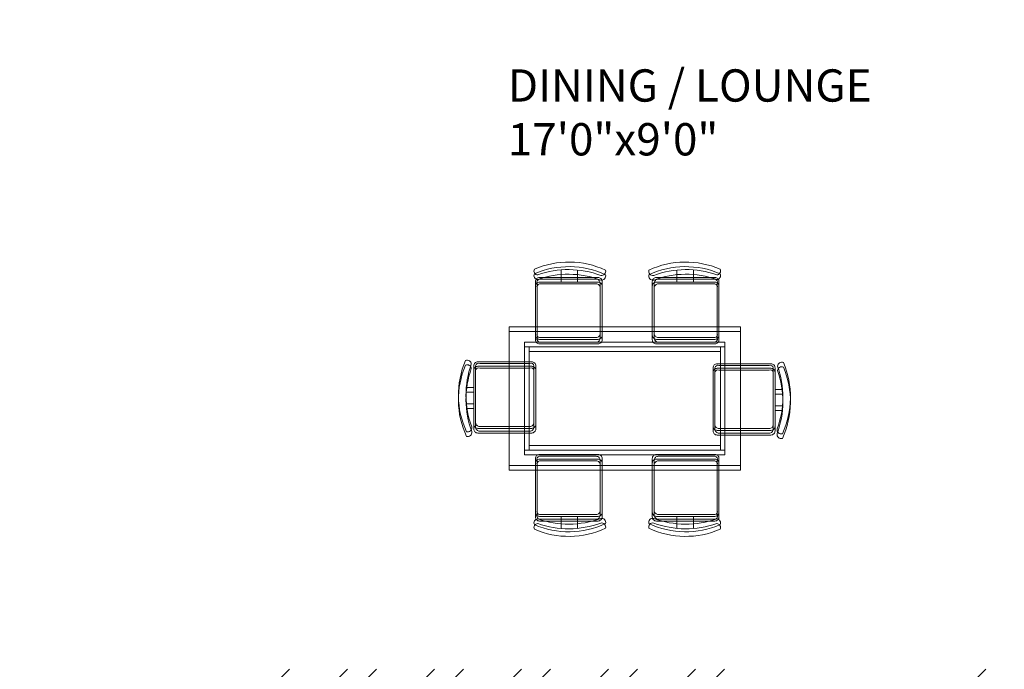
# Model space of a CAD drawing. Units: inches. Extents: x 963 to 2075, y 289 to 2657.
# Tile 55 of 98: x 1663 to 1815, y 1714 to 1814. Entities that reach past the tile are written whole.
import ezdxf

# ---------------------------------------------------------------- set-up
doc = ezdxf.new("R2010")
doc.units = ezdxf.units.IN
for name, color, linetype, lineweight in [('A-AREA-IDEN', 7, 'Continuous', 18), ('A-FURN', 8, 'Continuous', 18), ('A-WALL-PATT', 8, 'Continuous', 13)]:
    doc.layers.add(name, color=color, linetype=linetype, lineweight=lineweight)
doc.styles.get("Standard").update_dxf_attribs({"font": 'arial.ttf'})

msp = doc.modelspace()

# ---------------------------------------------------------------- hatches: boundary and pattern name
at = {"layer": 'A-WALL-PATT'}
h = msp.add_hatch(dxfattribs=at)
h.set_pattern_fill('ANSI32', color=256)
h.paths.add_polyline_path([(1296.92, 2558.32), (1203.92, 2558.32), (1203.92, 2493.82), (1191.53, 2493.82), (1191.53, 2489.32), (1211.06, 2489.32), (1211.06, 2492.02), (1211.06, 2493.82), (1208.42, 2493.82), (1208.42, 2553.82), (1292.42, 2553.82), (1292.42, 2538.86), (1296.92, 2538.86)])
h.paths.add_polyline_path([(1442.42, 2558.32), (1349.42, 2558.32), (1349.42, 2538.94), (1353.92, 2538.94), (1353.92, 2553.82), (1437.92, 2553.82), (1437.92, 2493.82), (1434.54, 2493.82), (1434.54, 2489.32), (1448.31, 2489.32), (1448.31, 2491.57), (1448.31, 2493.82), (1442.42, 2493.82)])
h.paths.add_polyline_path([(1415.55, 2491.57), (1415.55, 2493.82), (1340.94, 2493.82), (1340.94, 2489.32), (1371.92, 2489.32), (1371.92, 2378.32), (1367.6, 2378.32), (1367.6, 2373.82), (1371.92, 2373.82), (1371.92, 2355.19), (1376.42, 2355.19), (1376.42, 2489.32), (1415.55, 2489.32)])
h.paths.add_polyline_path([(1304.94, 2491.57), (1304.94, 2493.82), (1296.92, 2493.82), (1296.92, 2514.86), (1292.42, 2514.86), (1292.42, 2493.82), (1232.81, 2493.82), (1232.81, 2489.32), (1256.42, 2489.32), (1256.42, 2327.32), (1253.71, 2327.32), (1253.71, 2322.82), (1328.42, 2322.82), (1328.42, 2331.15), (1323.92, 2331.15), (1323.92, 2327.32), (1260.92, 2327.32), (1260.92, 2373.82), (1323.92, 2373.82), (1323.92, 2357.81), (1328.42, 2357.81), (1328.42, 2373.82), (1346.01, 2373.82), (1346.01, 2376.07), (1346.01, 2378.32), (1260.92, 2378.32), (1260.92, 2489.32), (1304.94, 2489.32)])
h.paths.add_polyline_path([(1226.65, 2327.32), (1124.42, 2327.32), (1124.42, 2347.45), (1119.92, 2347.45), (1119.92, 2322.82), (1163.42, 2322.82), (1163.42, 2305.43), (1165.67, 2305.43), (1167.92, 2305.43), (1167.92, 2322.82), (1226.65, 2322.82), (1226.65, 2325.07)])
h.paths.add_polyline_path([(1095.92, 2489.32), (1124.42, 2489.32), (1131.53, 2489.32), (1131.53, 2491.57), (1131.53, 2493.82), (1119.92, 2493.82), (1091.42, 2493.82), (1091.42, 2417.32), (1095.92, 2417.32), (1119.92, 2417.32), (1119.92, 2407.45), (1124.42, 2407.45), (1124.42, 2421.82), (1095.92, 2421.82)])
h.paths.add_polyline_path([(1512.92, 2558.32), (1508.42, 2558.32), (1508.42, 2493.82), (1503.4, 2493.82), (1503.4, 2489.32), (1508.42, 2489.32), (1508.42, 2327.32), (1376.42, 2327.32), (1376.42, 2330.27), (1371.92, 2330.27), (1371.92, 2298.74), (1376.42, 2298.74), (1376.42, 2322.82), (1508.42, 2322.82), (1508.42, 2165.32), (1504.26, 2165.32), (1504.26, 2160.82), (1508.42, 2160.82), (1508.42, 2108.32), (1512.92, 2108.32), (1512.92, 2160.82), (1516.18, 2160.82), (1516.18, 2163.07), (1516.18, 2165.32), (1512.92, 2165.32), (1512.92, 2322.82), (1644.92, 2322.82), (1644.92, 2298.74), (1649.42, 2298.74), (1649.42, 2322.82), (1649.42, 2330.94), (1647.17, 2330.94), (1644.92, 2330.94), (1644.92, 2327.32), (1512.92, 2327.32), (1512.92, 2489.32), (1516.76, 2489.32), (1516.76, 2491.57), (1516.76, 2493.82), (1512.92, 2493.82)])
h.paths.add_polyline_path([(1671.92, 2558.32), (1578.92, 2558.32), (1578.92, 2493.82), (1573.53, 2493.82), (1573.53, 2489.32), (1586.54, 2489.32), (1586.54, 2491.57), (1586.54, 2493.82), (1583.42, 2493.82), (1583.42, 2553.82), (1667.42, 2553.82), (1667.42, 2541.11), (1671.92, 2541.11)])
h.paths.add_polyline_path([(1681.26, 2493.82), (1671.92, 2493.82), (1671.92, 2517.11), (1667.42, 2517.11), (1667.42, 2493.82), (1610.22, 2493.82), (1610.22, 2489.32), (1644.92, 2489.32), (1644.92, 2357.87), (1649.42, 2357.87), (1649.42, 2373.82), (1652.2, 2373.82), (1652.2, 2375.83), (1652.2, 2378.32), (1649.42, 2378.32), (1649.42, 2489.32), (1681.26, 2489.32), (1681.26, 2491.57)])
h.paths.add_polyline_path([(1821.92, 2558.32), (1728.92, 2558.32), (1728.92, 2541), (1733.42, 2541), (1733.42, 2553.82), (1817.42, 2553.82), (1817.42, 2493.82), (1813.51, 2493.82), (1813.51, 2489.32), (1830.08, 2489.32), (1830.08, 2491.57), (1830.08, 2493.82), (1821.92, 2493.82)])
h.paths.add_polyline_path([(1794.24, 2493.82), (1717.26, 2493.82), (1717.26, 2489.32), (1760.42, 2489.32), (1760.42, 2378.32), (1674.4, 2378.32), (1674.4, 2373.82), (1692.92, 2373.82), (1692.92, 2356.95), (1697.42, 2356.95), (1697.42, 2373.82), (1760.42, 2373.82), (1760.42, 2327.32), (1697.42, 2327.32), (1697.42, 2333.34), (1692.92, 2333.34), (1692.92, 2322.82), (1768.04, 2322.82), (1768.04, 2325.07), (1768.04, 2327.32), (1764.92, 2327.32), (1764.92, 2489.32), (1794.24, 2489.32)])
h.paths.add_polyline_path([(1733.42, 2517), (1728.92, 2517), (1728.92, 2493.82), (1733.42, 2493.82)], flags=17)
h.paths.add_polyline_path([(1929.92, 2493.82), (1890.08, 2493.82), (1890.08, 2489.32), (1896.92, 2489.32), (1925.42, 2489.32), (1925.42, 2421.82), (1896.92, 2421.82), (1896.92, 2408.32), (1901.42, 2408.32), (1901.42, 2417.32), (1925.42, 2417.32), (1929.92, 2417.32)])
h.paths.add_polyline_path([(1901.42, 2348.32), (1896.92, 2348.32), (1896.92, 2327.32), (1800.42, 2327.32), (1800.42, 2322.82), (1853.42, 2322.82), (1853.42, 2309.45), (1857.92, 2309.45), (1857.92, 2322.82), (1901.42, 2322.82)])
h.paths.add_polyline_path([(1857.92, 2249.45), (1853.42, 2249.45), (1853.42, 2214.82), (1686.31, 2214.82), (1686.31, 2210.32), (1853.42, 2210.32), (1853.42, 2202.13), (1857.92, 2202.13), (1857.92, 2210.32)])
h.paths.add_polyline_path([(1857.92, 2142.13), (1853.42, 2142.13), (1853.42, 2115.42), (1841.42, 2115.42), (1841.42, 2088.53), (1841.42, 2046.95), (1845.92, 2046.95), (1845.92, 2110.92), (1905.92, 2110.92), (1905.92, 2092.52), (1910.42, 2092.52), (1910.42, 2115.42), (1857.92, 2115.42)])
h.paths.add_polyline_path([(1532.44, 1482.34), (1573.46, 1482.34), (1573.46, 1501), (1532.44, 1501)], flags=9)
h.paths.add_polyline_path([(1438.66, 1486.3), (1479.68, 1486.3), (1479.68, 1504.96), (1438.66, 1504.96)], flags=9)
h.paths.add_polyline_path([(1411.22, 1365.31), (1659.14, 1365.31), (1659.14, 1402.4), (1411.22, 1402.4)], flags=9)
h.paths.add_polyline_path([(1185.67, 2296.3), (1248.16, 2296.3), (1248.16, 2314.95), (1185.67, 2314.95)], flags=9)
h.paths.add_polyline_path([(1177.31, 2187.35), (1216.15, 2187.35), (1216.15, 2206.01), (1177.31, 2206.01)], flags=9)
h.paths.add_polyline_path([(1295.1, 1602.08), (1328.26, 1602.08), (1328.26, 1620.74), (1295.1, 1620.74)], flags=9)
h.paths.add_polyline_path([(1525.13, 2005.99), (1558.39, 2005.99), (1558.39, 2024.65), (1525.13, 2024.65)], flags=9)
h.paths.add_polyline_path([(1459.61, 1977.13), (1472.19, 1977.13), (1472.19, 1987.43), (1459.61, 1987.43)], flags=9)
h.paths.add_polyline_path([(1467.81, 2053.68), (1480.02, 2053.68), (1480.02, 2063.98), (1467.81, 2063.98)], flags=9)
h.paths.add_polyline_path([(1555.18, 2119.02), (1584.56, 2119.02), (1584.56, 2137.68), (1555.18, 2137.68)], flags=25)
h.paths.add_polyline_path([(1405.39, 2115.29), (1444.48, 2115.29), (1444.48, 2133.95), (1405.39, 2133.95)], flags=25)
h.paths.add_polyline_path([(1698.48, 2004.26), (1727.69, 2004.26), (1727.69, 2022.92), (1698.48, 2022.92)], flags=9)
h.paths.add_polyline_path([(1612.16, 1972.86), (1629.02, 1972.86), (1629.02, 1983.16), (1612.16, 1983.16)], flags=9)
h.paths.add_polyline_path([(1608.29, 2060.04), (1625.15, 2060.04), (1625.15, 2070.34), (1608.29, 2070.34)], flags=9)
h.paths.add_polyline_path([(1527.95, 1684.4), (1566.79, 1684.4), (1566.79, 1703.06), (1527.95, 1703.06)], flags=9)
h.paths.add_polyline_path([(1422.79, 1683.59), (1461.63, 1683.59), (1461.63, 1702.25), (1422.79, 1702.25)], flags=9)
h.paths.add_polyline_path([(1531.26, 1732.46), (1574.01, 1732.46), (1574.01, 1751.12), (1531.26, 1751.12)], flags=9)
h.paths.add_polyline_path([(1402.87, 1732.85), (1439.8, 1732.85), (1439.8, 1751.5), (1402.87, 1751.5)], flags=9)
h.paths.add_polyline_path([(1243.12, 1923.13), (1281.96, 1923.13), (1281.96, 1941.79), (1243.12, 1941.79)], flags=9)
h.paths.add_polyline_path([(1181.75, 1792.27), (1244.24, 1792.27), (1244.24, 1810.93), (1181.75, 1810.93)], flags=9)
h.paths.add_polyline_path([(1265.82, 1670.3), (1316.07, 1670.3), (1316.07, 1688.96), (1265.82, 1688.96)], flags=9)
h.paths.add_polyline_path([(1140.26, 1676.05), (1179.1, 1676.05), (1179.1, 1694.71), (1140.26, 1694.71)], flags=9)
h.paths.add_polyline_path([(1107.49, 1490.89), (1143.37, 1490.89), (1143.37, 1509.55), (1107.49, 1509.55)], flags=9)
h.paths.add_polyline_path([(1217.58, 1483.9), (1246.74, 1483.9), (1246.74, 1502.56), (1217.58, 1502.56)], flags=9)
h.paths.add_polyline_path([(1389.21, 1486.92), (1418.37, 1486.92), (1418.37, 1505.58), (1389.21, 1505.58)], flags=9)
h.paths.add_polyline_path([(1672.21, 1602.08), (1705.37, 1602.08), (1705.37, 1620.74), (1672.21, 1620.74)], flags=9)
h.paths.add_polyline_path([(1752.08, 1522.64), (1781.24, 1522.64), (1781.24, 1541.3), (1752.08, 1541.3)], flags=9)
h.paths.add_polyline_path([(1848.27, 1491.26), (1884.16, 1491.26), (1884.16, 1509.92), (1848.27, 1509.92)], flags=9)
h.paths.add_polyline_path([(1822.47, 1685.62), (1861.31, 1685.62), (1861.31, 1704.28), (1822.47, 1704.28)], flags=9)
h.paths.add_polyline_path([(1713.19, 1672.23), (1763.44, 1672.23), (1763.44, 1690.89), (1713.19, 1690.89)], flags=9)
h.paths.add_polyline_path([(1736.62, 1790.58), (1799.11, 1790.58), (1799.11, 1809.24), (1736.62, 1809.24)], flags=9)
h.paths.add_polyline_path([(1691.49, 1916.36), (1730.33, 1916.36), (1730.33, 1935.01), (1691.49, 1935.01)], flags=9)
h.paths.add_polyline_path([(1764.87, 1973.92), (1794.31, 1973.92), (1794.31, 1992.58), (1764.87, 1992.58)], flags=9)
h.paths.add_polyline_path([(1767.85, 2034.02), (1797.29, 2034.02), (1797.29, 2052.67), (1767.85, 2052.67)], flags=9)
h.paths.add_polyline_path([(1851.59, 2060.33), (1880.75, 2060.33), (1880.75, 2078.99), (1851.59, 2078.99)], flags=25)
h.paths.add_polyline_path([(1688.49, 2086.87), (1727.33, 2086.87), (1727.33, 2105.53), (1688.49, 2105.53)], flags=9)
h.paths.add_polyline_path([(1537.74, 2293.58), (1580.49, 2293.58), (1580.49, 2312.24), (1537.74, 2312.24)], flags=25)
h.paths.add_polyline_path([(1425.59, 2296.11), (1468.34, 2296.11), (1468.34, 2314.77), (1425.59, 2314.77)], flags=25)
h.paths.add_polyline_path([(1278.52, 2004.18), (1307.72, 2004.18), (1307.72, 2022.84), (1278.52, 2022.84)], flags=9)
h.paths.add_polyline_path([(1193.28, 1973.63), (1222.72, 1973.63), (1222.72, 1992.29), (1193.28, 1992.29)], flags=9)
h.paths.add_polyline_path([(1192.41, 2040.58), (1221.84, 2040.58), (1221.84, 2059.23), (1192.41, 2059.23)], flags=9)
h.paths.add_polyline_path([(1130.6, 1951.39), (1159.76, 1951.39), (1159.76, 1970.05), (1130.6, 1970.05)], flags=9)
h.paths.add_polyline_path([(1132.83, 2052.49), (1161.98, 2052.49), (1161.98, 2071.15), (1132.83, 2071.15)], flags=9)
h.paths.add_polyline_path([(1265.13, 2334.62), (1315.38, 2334.62), (1315.38, 2353.28), (1265.13, 2353.28)], flags=25)
h.paths.add_polyline_path([(1136.74, 2330.79), (1175.58, 2330.79), (1175.58, 2349.44), (1136.74, 2349.44)], flags=9)
h.paths.add_polyline_path([(1287.42, 2417.2), (1320.58, 2417.2), (1320.58, 2435.86), (1287.42, 2435.86)], flags=25)
h.paths.add_polyline_path([(1430.99, 2329.16), (1469.83, 2329.16), (1469.83, 2347.82), (1430.99, 2347.82)], flags=25)
h.paths.add_polyline_path([(1525.42, 2329.21), (1564.26, 2329.21), (1564.26, 2347.87), (1525.42, 2347.87)], flags=25)
h.paths.add_polyline_path([(1684.52, 2382.8), (1717.68, 2382.8), (1717.68, 2401.46), (1684.52, 2401.46)], flags=25)
h.paths.add_polyline_path([(1704.81, 2340.29), (1755.05, 2340.29), (1755.05, 2358.95), (1704.81, 2358.95)], flags=25)
h.paths.add_polyline_path([(1694.11, 2287.76), (1756.6, 2287.76), (1756.6, 2306.41), (1694.11, 2306.41)], flags=9)
h.paths.add_polyline_path([(1815.78, 2329.86), (1854.62, 2329.86), (1854.62, 2348.52), (1815.78, 2348.52)], flags=9)
h.paths.add_polyline_path([(1842.87, 2514.26), (1878.76, 2514.26), (1878.76, 2532.91), (1842.87, 2532.91)], flags=9)
h.paths.add_polyline_path([(1769.51, 2531.45), (1798.67, 2531.45), (1798.67, 2550.1), (1769.51, 2550.1)], flags=25)
h.paths.add_polyline_path([(1594.77, 2518.47), (1623.93, 2518.47), (1623.93, 2537.13), (1594.77, 2537.13)], flags=25)
h.paths.add_polyline_path([(1520.72, 2516.18), (1556.61, 2516.18), (1556.61, 2534.84), (1520.72, 2534.84)], flags=25)
h.paths.add_polyline_path([(1464.46, 2516.69), (1500.34, 2516.69), (1500.34, 2535.35), (1464.46, 2535.35)], flags=25)
h.paths.add_polyline_path([(1365.7, 2528.97), (1394.85, 2528.97), (1394.85, 2547.63), (1365.7, 2547.63)], flags=25)
h.paths.add_polyline_path([(1222.84, 2516.23), (1252, 2516.23), (1252, 2534.89), (1222.84, 2534.89)], flags=25)
h.paths.add_polyline_path([(1104.55, 2509.6), (1140.43, 2509.6), (1140.43, 2528.26), (1104.55, 2528.26)], flags=9)
h = msp.add_hatch(dxfattribs=at)
h.set_pattern_fill('ANSI32', color=256)
h.paths.add_polyline_path([(1335.97, 2212.57), (1335.97, 2214.82), (1167.92, 2214.82), (1167.92, 2245.43), (1163.42, 2245.43), (1163.42, 2210.32), (1163.42, 2194.81), (1167.92, 2194.81), (1167.92, 2210.32), (1335.97, 2210.32)])
h.paths.add_polyline_path([(1532.44, 1482.34), (1573.46, 1482.34), (1573.46, 1501), (1532.44, 1501)], flags=9)
h.paths.add_polyline_path([(1438.66, 1486.3), (1479.68, 1486.3), (1479.68, 1504.96), (1438.66, 1504.96)], flags=9)
h.paths.add_polyline_path([(1411.22, 1365.31), (1659.14, 1365.31), (1659.14, 1402.4), (1411.22, 1402.4)], flags=9)
h.paths.add_polyline_path([(1185.67, 2296.3), (1248.16, 2296.3), (1248.16, 2314.95), (1185.67, 2314.95)], flags=9)
h.paths.add_polyline_path([(1177.31, 2187.35), (1216.15, 2187.35), (1216.15, 2206.01), (1177.31, 2206.01)], flags=9)
h.paths.add_polyline_path([(1295.1, 1602.08), (1328.26, 1602.08), (1328.26, 1620.74), (1295.1, 1620.74)], flags=9)
h.paths.add_polyline_path([(1525.13, 2005.99), (1558.39, 2005.99), (1558.39, 2024.65), (1525.13, 2024.65)], flags=9)
h.paths.add_polyline_path([(1459.61, 1977.13), (1472.19, 1977.13), (1472.19, 1987.43), (1459.61, 1987.43)], flags=9)
h.paths.add_polyline_path([(1467.81, 2053.68), (1480.02, 2053.68), (1480.02, 2063.98), (1467.81, 2063.98)], flags=9)
h.paths.add_polyline_path([(1555.18, 2119.02), (1584.56, 2119.02), (1584.56, 2137.68), (1555.18, 2137.68)], flags=9)
h.paths.add_polyline_path([(1405.39, 2115.29), (1444.48, 2115.29), (1444.48, 2133.95), (1405.39, 2133.95)], flags=9)
h.paths.add_polyline_path([(1698.48, 2004.26), (1727.69, 2004.26), (1727.69, 2022.92), (1698.48, 2022.92)], flags=9)
h.paths.add_polyline_path([(1612.16, 1972.86), (1629.02, 1972.86), (1629.02, 1983.16), (1612.16, 1983.16)], flags=9)
h.paths.add_polyline_path([(1608.29, 2060.04), (1625.15, 2060.04), (1625.15, 2070.34), (1608.29, 2070.34)], flags=9)
h.paths.add_polyline_path([(1527.95, 1684.4), (1566.79, 1684.4), (1566.79, 1703.06), (1527.95, 1703.06)], flags=9)
h.paths.add_polyline_path([(1422.79, 1683.59), (1461.63, 1683.59), (1461.63, 1702.25), (1422.79, 1702.25)], flags=9)
h.paths.add_polyline_path([(1531.26, 1732.46), (1574.01, 1732.46), (1574.01, 1751.12), (1531.26, 1751.12)], flags=9)
h.paths.add_polyline_path([(1402.87, 1732.85), (1439.8, 1732.85), (1439.8, 1751.5), (1402.87, 1751.5)], flags=9)
h.paths.add_polyline_path([(1243.12, 1923.13), (1281.96, 1923.13), (1281.96, 1941.79), (1243.12, 1941.79)], flags=9)
h.paths.add_polyline_path([(1181.75, 1792.27), (1244.24, 1792.27), (1244.24, 1810.93), (1181.75, 1810.93)], flags=9)
h.paths.add_polyline_path([(1265.82, 1670.3), (1316.07, 1670.3), (1316.07, 1688.96), (1265.82, 1688.96)], flags=9)
h.paths.add_polyline_path([(1140.26, 1676.05), (1179.1, 1676.05), (1179.1, 1694.71), (1140.26, 1694.71)], flags=9)
h.paths.add_polyline_path([(1107.49, 1490.89), (1143.37, 1490.89), (1143.37, 1509.55), (1107.49, 1509.55)], flags=9)
h.paths.add_polyline_path([(1217.58, 1483.9), (1246.74, 1483.9), (1246.74, 1502.56), (1217.58, 1502.56)], flags=9)
h.paths.add_polyline_path([(1389.21, 1486.92), (1418.37, 1486.92), (1418.37, 1505.58), (1389.21, 1505.58)], flags=9)
h.paths.add_polyline_path([(1672.21, 1602.08), (1705.37, 1602.08), (1705.37, 1620.74), (1672.21, 1620.74)], flags=9)
h.paths.add_polyline_path([(1752.08, 1522.64), (1781.24, 1522.64), (1781.24, 1541.3), (1752.08, 1541.3)], flags=9)
h.paths.add_polyline_path([(1848.27, 1491.26), (1884.16, 1491.26), (1884.16, 1509.92), (1848.27, 1509.92)], flags=9)
h.paths.add_polyline_path([(1822.47, 1685.62), (1861.31, 1685.62), (1861.31, 1704.28), (1822.47, 1704.28)], flags=9)
h.paths.add_polyline_path([(1713.19, 1672.23), (1763.44, 1672.23), (1763.44, 1690.89), (1713.19, 1690.89)], flags=9)
h.paths.add_polyline_path([(1736.62, 1790.58), (1799.11, 1790.58), (1799.11, 1809.24), (1736.62, 1809.24)], flags=9)
h.paths.add_polyline_path([(1691.49, 1916.36), (1730.33, 1916.36), (1730.33, 1935.01), (1691.49, 1935.01)], flags=9)
h.paths.add_polyline_path([(1764.87, 1973.92), (1794.31, 1973.92), (1794.31, 1992.58), (1764.87, 1992.58)], flags=9)
h.paths.add_polyline_path([(1767.85, 2034.02), (1797.29, 2034.02), (1797.29, 2052.67), (1767.85, 2052.67)], flags=9)
h.paths.add_polyline_path([(1851.59, 2060.33), (1880.75, 2060.33), (1880.75, 2078.99), (1851.59, 2078.99)], flags=9)
h.paths.add_polyline_path([(1688.49, 2086.87), (1727.33, 2086.87), (1727.33, 2105.53), (1688.49, 2105.53)], flags=9)
h.paths.add_polyline_path([(1537.74, 2293.58), (1580.49, 2293.58), (1580.49, 2312.24), (1537.74, 2312.24)], flags=9)
h.paths.add_polyline_path([(1425.59, 2296.11), (1468.34, 2296.11), (1468.34, 2314.77), (1425.59, 2314.77)], flags=9)
h.paths.add_polyline_path([(1278.52, 2004.18), (1307.72, 2004.18), (1307.72, 2022.84), (1278.52, 2022.84)], flags=9)
h.paths.add_polyline_path([(1193.28, 1973.63), (1222.72, 1973.63), (1222.72, 1992.29), (1193.28, 1992.29)], flags=9)
h.paths.add_polyline_path([(1192.41, 2040.58), (1221.84, 2040.58), (1221.84, 2059.23), (1192.41, 2059.23)], flags=9)
h.paths.add_polyline_path([(1130.6, 1951.39), (1159.76, 1951.39), (1159.76, 1970.05), (1130.6, 1970.05)], flags=9)
h.paths.add_polyline_path([(1132.83, 2052.49), (1161.98, 2052.49), (1161.98, 2071.15), (1132.83, 2071.15)], flags=9)
h.paths.add_polyline_path([(1265.13, 2334.62), (1315.38, 2334.62), (1315.38, 2353.28), (1265.13, 2353.28)], flags=9)
h.paths.add_polyline_path([(1136.74, 2330.79), (1175.58, 2330.79), (1175.58, 2349.44), (1136.74, 2349.44)], flags=9)
h.paths.add_polyline_path([(1287.42, 2417.2), (1320.58, 2417.2), (1320.58, 2435.86), (1287.42, 2435.86)], flags=9)
h.paths.add_polyline_path([(1430.99, 2329.16), (1469.83, 2329.16), (1469.83, 2347.82), (1430.99, 2347.82)], flags=9)
h.paths.add_polyline_path([(1525.42, 2329.21), (1564.26, 2329.21), (1564.26, 2347.87), (1525.42, 2347.87)], flags=9)
h.paths.add_polyline_path([(1684.52, 2382.8), (1717.68, 2382.8), (1717.68, 2401.46), (1684.52, 2401.46)], flags=9)
h.paths.add_polyline_path([(1704.81, 2340.29), (1755.05, 2340.29), (1755.05, 2358.95), (1704.81, 2358.95)], flags=9)
h.paths.add_polyline_path([(1694.11, 2287.76), (1756.6, 2287.76), (1756.6, 2306.41), (1694.11, 2306.41)], flags=9)
h.paths.add_polyline_path([(1815.78, 2329.86), (1854.62, 2329.86), (1854.62, 2348.52), (1815.78, 2348.52)], flags=9)
h.paths.add_polyline_path([(1842.87, 2514.26), (1878.76, 2514.26), (1878.76, 2532.91), (1842.87, 2532.91)], flags=9)
h.paths.add_polyline_path([(1769.51, 2531.45), (1798.67, 2531.45), (1798.67, 2550.1), (1769.51, 2550.1)], flags=9)
h.paths.add_polyline_path([(1594.77, 2518.47), (1623.93, 2518.47), (1623.93, 2537.13), (1594.77, 2537.13)], flags=9)
h.paths.add_polyline_path([(1520.72, 2516.18), (1556.61, 2516.18), (1556.61, 2534.84), (1520.72, 2534.84)], flags=9)
h.paths.add_polyline_path([(1464.46, 2516.69), (1500.34, 2516.69), (1500.34, 2535.35), (1464.46, 2535.35)], flags=9)
h.paths.add_polyline_path([(1365.7, 2528.97), (1394.85, 2528.97), (1394.85, 2547.63), (1365.7, 2547.63)], flags=9)
h.paths.add_polyline_path([(1222.84, 2516.23), (1252, 2516.23), (1252, 2534.89), (1222.84, 2534.89)], flags=9)
h.paths.add_polyline_path([(1104.55, 2509.6), (1140.43, 2509.6), (1140.43, 2528.26), (1104.55, 2528.26)], flags=9)
h = msp.add_hatch(dxfattribs=at)
h.set_pattern_fill('ANSI32', color=256)
h.paths.add_polyline_path([(1910.42, 1929.42), (1910.42, 1963.51), (1905.92, 1963.51), (1905.92, 1929.42), (1845.92, 1929.42), (1845.92, 1993.37), (1843.67, 1993.37), (1841.42, 1993.37), (1841.42, 1951.16), (1841.42, 1924.92), (1853.42, 1924.92), (1853.42, 1913.07), (1857.92, 1913.07), (1857.92, 1924.92), (1910.42, 1924.92)])
h.paths.add_polyline_path([(1857.92, 1853.07), (1853.42, 1853.07), (1853.42, 1826.32), (1841.42, 1826.32), (1674.48, 1826.32), (1674.48, 1821.82), (1853.42, 1821.82), (1857.92, 1821.82)])
h.paths.add_polyline_path([(1857.92, 1821.82), (1853.42, 1821.82), (1853.42, 1807.79), (1857.92, 1807.79)])
h.paths.add_polyline_path([(1857.92, 1747.79), (1853.42, 1747.79), (1853.42, 1713.82), (1809.34, 1713.82), (1809.34, 1709.32), (1905.92, 1709.32), (1905.92, 1688.32), (1910.42, 1688.32), (1910.42, 1713.82), (1857.92, 1713.82)])
h.paths.add_polyline_path([(1830.92, 1542.82), (1837.43, 1542.82), (1837.43, 1545.07), (1837.43, 1547.32), (1823.42, 1547.32), (1823.42, 1545.07), (1823.42, 1542.82), (1826.42, 1542.82), (1826.42, 1482.82), (1742.42, 1482.82), (1742.42, 1505.39), (1737.92, 1505.39), (1737.92, 1478.32), (1830.92, 1478.32)])
h.paths.add_polyline_path([(1938.92, 1619.32), (1934.42, 1619.32), (1910.42, 1619.32), (1910.42, 1628.32), (1908.17, 1628.32), (1905.92, 1628.32), (1905.92, 1614.82), (1934.42, 1614.82), (1934.42, 1547.32), (1905.92, 1547.32), (1899.59, 1547.32), (1899.59, 1542.82), (1910.42, 1542.82), (1938.92, 1542.82)])
h.paths.add_polyline_path([(1803.68, 1547.32), (1773.92, 1547.32), (1773.92, 1709.32), (1777.76, 1709.32), (1777.76, 1713.82), (1701.92, 1713.82), (1701.92, 1697.8), (1706.42, 1697.8), (1706.42, 1709.32), (1769.42, 1709.32), (1769.42, 1662.82), (1706.42, 1662.82), (1706.42, 1674.38), (1701.92, 1674.38), (1701.92, 1662.82), (1675.67, 1662.82), (1675.67, 1658.32), (1769.42, 1658.32), (1769.42, 1547.32), (1729.17, 1547.32), (1729.17, 1542.82), (1737.92, 1542.82), (1737.92, 1529.39), (1742.42, 1529.39), (1742.42, 1542.82), (1803.68, 1542.82)])
h.paths.add_polyline_path([(1595.42, 1542.82), (1599.24, 1542.82), (1599.24, 1547.32), (1584.36, 1547.32), (1584.36, 1542.82), (1590.92, 1542.82), (1590.92, 1436.32), (1595.42, 1436.32), (1595.42, 1440.82)])
h.paths.add_polyline_path([(1693.17, 1547.32), (1649.42, 1547.32), (1649.42, 1658.32), (1652.1, 1658.32), (1652.1, 1660.57), (1652.1, 1662.82), (1649.42, 1662.82), (1649.42, 1680.94), (1647.17, 1680.94), (1644.92, 1680.94), (1644.92, 1547.32), (1622.42, 1547.32), (1622.42, 1545.07), (1622.42, 1542.82), (1649.42, 1542.82), (1679.42, 1542.82), (1679.42, 1529.85), (1681.67, 1529.85), (1683.92, 1529.85), (1683.92, 1542.82), (1693.17, 1542.82), (1693.17, 1545.07)])
h.paths.add_polyline_path([(1683.92, 1505.85), (1679.42, 1505.85), (1679.42, 1483.8), (1595.42, 1483.8), (1595.42, 1479.3), (1683.92, 1479.3)])
h.paths.add_polyline_path([(1402.99, 1547.32), (1376.42, 1547.32), (1376.42, 1675.89), (1374.17, 1675.89), (1371.92, 1675.89), (1371.92, 1662.82), (1368.88, 1662.82), (1368.88, 1658.32), (1371.92, 1658.32), (1371.92, 1547.32), (1335.46, 1547.32), (1335.46, 1542.82), (1337.42, 1542.82), (1337.42, 1526.73), (1341.92, 1526.73), (1341.92, 1542.82), (1371.92, 1542.82), (1402.99, 1542.82)])

# ---------------------------------------------------------------- linework, layer by layer
at = {"layer": 'A-FURN'}
for points in [[(1743.26, 1774.91, -0.175809), (1753.01, 1774.84, 0.578392), (1753.75, 1775.65, 0.214524), (1742.74, 1775.8, 0.552014), (1743.26, 1774.91, -0.065079)], [(1743.26, 1774.91, -0.175809), (1753.01, 1774.84, 0.578392), (1753.75, 1775.65, 0.214524), (1742.74, 1775.8, 0.552014), (1743.26, 1774.91, -0.065079)], [(1743.26, 1774.2, -0.175809), (1753.01, 1774.12, 0.578392), (1753.75, 1774.94, 0.214524), (1742.74, 1775.08, 0.552014), (1743.26, 1774.2, -0.065079)], [(1743.26, 1774.2, -0.175809), (1753.01, 1774.12, 0.578392), (1753.75, 1774.94, 0.214524), (1742.74, 1775.08, 0.552014), (1743.26, 1774.2, -0.065079)], [(1749.41, 1774.52), (1749.41, 1775.67, -0.064759)], [(1749.41, 1774.52), (1749.41, 1775.67, -0.064759)], [(1761.22, 1774.84, -0.578392), (1760.48, 1775.65, -0.214524), (1771.49, 1775.8, -0.552014), (1770.97, 1774.91, 0.175809), (1761.22, 1774.84)], [(1761.22, 1774.84, -0.578392), (1760.48, 1775.65, -0.214524), (1771.49, 1775.8, -0.552014), (1770.97, 1774.91, 0.175809), (1761.22, 1774.84)], [(1761.22, 1774.12, -0.578392), (1760.48, 1774.94, -0.214524), (1771.49, 1775.08, -0.552014), (1770.97, 1774.2, 0.175809), (1761.22, 1774.12)], [(1761.22, 1774.12, -0.578392), (1760.48, 1774.94, -0.214524), (1771.49, 1775.08, -0.552014), (1770.97, 1774.2, 0.175809), (1761.22, 1774.12)], [(1764.82, 1774.52), (1764.82, 1775.67, 0.064759)], [(1764.82, 1774.52), (1764.82, 1775.67, 0.064759)], [(1752.6, 1774.52), (1743.54, 1774.52, 0.414214), (1742.91, 1773.89), (1742.91, 1765.56, 0.414214), (1743.54, 1764.93), (1752.6, 1764.93, 0.414214), (1753.23, 1765.56), (1753.23, 1773.89, 0.414214), (1752.6, 1774.52)], [(1752.6, 1774.52), (1743.54, 1774.52, 0.414214), (1742.91, 1773.89), (1742.91, 1765.56, 0.414214), (1743.54, 1764.93), (1752.6, 1764.93, 0.414214), (1753.23, 1765.56), (1753.23, 1773.89, 0.414214), (1752.6, 1774.52)], [(1749.41, 1773.81), (1749.41, 1774.95, -0.064759)], [(1749.41, 1773.81), (1749.41, 1774.95, -0.064759)], [(1770.69, 1774.52, -0.414214), (1771.32, 1773.89), (1771.32, 1765.56, -0.414214), (1770.69, 1764.93), (1761.63, 1764.93, -0.414214), (1761, 1765.56), (1761, 1773.89, -0.414214), (1761.63, 1774.52), (1770.69, 1774.52)], [(1770.69, 1774.52, -0.414214), (1771.32, 1773.89), (1771.32, 1765.56, -0.414214), (1770.69, 1764.93), (1761.63, 1764.93, -0.414214), (1761, 1765.56), (1761, 1773.89, -0.414214), (1761.63, 1774.52), (1770.69, 1774.52)], [(1764.82, 1773.81), (1764.82, 1774.95, 0.064759)], [(1764.82, 1773.81), (1764.82, 1774.95, 0.064759)], [(1752.6, 1773.81), (1743.54, 1773.81, 0.414214), (1742.91, 1773.17), (1742.91, 1764.85, 0.414214), (1743.54, 1764.21), (1752.6, 1764.21, 0.414214), (1753.23, 1764.85), (1753.23, 1773.17, 0.414214), (1752.6, 1773.81)], [(1752.6, 1773.81), (1743.54, 1773.81, 0.414214), (1742.91, 1773.17), (1742.91, 1764.85, 0.414214), (1743.54, 1764.21), (1752.6, 1764.21, 0.414214), (1753.23, 1764.85), (1753.23, 1773.17, 0.414214), (1752.6, 1773.81)], [(1770.69, 1773.81, -0.414214), (1771.32, 1773.17), (1771.32, 1764.85, -0.414214), (1770.69, 1764.21), (1761.63, 1764.21, -0.414214), (1761, 1764.85), (1761, 1773.17, -0.414214), (1761.63, 1773.81), (1770.69, 1773.81)], [(1770.69, 1773.81, -0.414214), (1771.32, 1773.17), (1771.32, 1764.85, -0.414214), (1770.69, 1764.21), (1761.63, 1764.21, -0.414214), (1761, 1764.85), (1761, 1773.17, -0.414214), (1761.63, 1773.81), (1770.69, 1773.81)], [(1733.05, 1751.36, -0.578392), (1732.24, 1750.62, -0.214524), (1732.09, 1761.63, -0.552014), (1732.98, 1761.11, 0.175809), (1733.05, 1751.36)], [(1733.05, 1751.36, -0.578392), (1732.24, 1750.62, -0.214524), (1732.09, 1761.63, -0.552014), (1732.98, 1761.11, 0.175809), (1733.05, 1751.36)], [(1733.05, 1750.64, -0.578392), (1732.24, 1749.9, -0.214524), (1732.09, 1760.91, -0.552014), (1732.98, 1760.4, 0.175809), (1733.05, 1750.64)], [(1733.05, 1750.64, -0.578392), (1732.24, 1749.9, -0.214524), (1732.09, 1760.91, -0.552014), (1732.98, 1760.4, 0.175809), (1733.05, 1750.64)], [(1733.37, 1760.83, -0.414214), (1734, 1761.46), (1742.33, 1761.46, -0.414214), (1742.96, 1760.83), (1742.96, 1751.77, -0.414214), (1742.33, 1751.14), (1734, 1751.14, -0.414214), (1733.37, 1751.77), (1733.37, 1760.83)], [(1733.37, 1760.83, -0.414214), (1734, 1761.46), (1742.33, 1761.46, -0.414214), (1742.96, 1760.83), (1742.96, 1751.77, -0.414214), (1742.33, 1751.14), (1734, 1751.14, -0.414214), (1733.37, 1751.77), (1733.37, 1760.83)], [(1733.37, 1760.11, -0.414214), (1734, 1760.75), (1742.33, 1760.75, -0.414214), (1742.96, 1760.11), (1742.96, 1751.06, -0.414214), (1742.33, 1750.42), (1734, 1750.42, -0.414214), (1733.37, 1751.06), (1733.37, 1760.11)], [(1733.37, 1760.11, -0.414214), (1734, 1760.75), (1742.33, 1760.75, -0.414214), (1742.96, 1760.11), (1742.96, 1751.06, -0.414214), (1742.33, 1750.42), (1734, 1750.42, -0.414214), (1733.37, 1751.06), (1733.37, 1760.11)], [(1780, 1760.52, 0.414214), (1779.37, 1761.15), (1771.04, 1761.15, 0.414214), (1770.41, 1760.52), (1770.41, 1751.46, 0.414214), (1771.04, 1750.83), (1779.37, 1750.83, 0.414214), (1780, 1751.46), (1780, 1760.52)], [(1780, 1760.52, 0.414214), (1779.37, 1761.15), (1771.04, 1761.15, 0.414214), (1770.41, 1760.52), (1770.41, 1751.46, 0.414214), (1771.04, 1750.83), (1779.37, 1750.83, 0.414214), (1780, 1751.46), (1780, 1760.52)], [(1780, 1759.8, 0.414214), (1779.37, 1760.44), (1771.04, 1760.44, 0.414214), (1770.41, 1759.8), (1770.41, 1750.75, 0.414214), (1771.04, 1750.11), (1779.37, 1750.11, 0.414214), (1780, 1750.75), (1780, 1759.8)], [(1780, 1759.8, 0.414214), (1779.37, 1760.44), (1771.04, 1760.44, 0.414214), (1770.41, 1759.8), (1770.41, 1750.75, 0.414214), (1771.04, 1750.11), (1779.37, 1750.11, 0.414214), (1780, 1750.75), (1780, 1759.8)], [(1780.39, 1760.8, -0.175809), (1780.32, 1751.05, 0.578392), (1781.13, 1750.31, 0.214524), (1781.28, 1761.32, 0.552014), (1780.39, 1760.8, -0.065079)], [(1780.39, 1760.8, -0.175809), (1780.32, 1751.05, 0.578392), (1781.13, 1750.31, 0.214524), (1781.28, 1761.32, 0.552014), (1780.39, 1760.8, -0.065079)], [(1780.39, 1760.09, -0.175809), (1780.32, 1750.33, 0.578392), (1781.13, 1749.59, 0.214524), (1781.28, 1760.6, 0.552014), (1780.39, 1760.09, -0.065079)], [(1780.39, 1760.09, -0.175809), (1780.32, 1750.33, 0.578392), (1781.13, 1749.59, 0.214524), (1781.28, 1760.6, 0.552014), (1780.39, 1760.09, -0.065079)], [(1733.37, 1754.95), (1732.22, 1754.95, 0.064759)], [(1733.37, 1754.95), (1732.22, 1754.95, 0.064759)], [(1733.37, 1754.24), (1732.22, 1754.24, 0.064759)], [(1733.37, 1754.24), (1732.22, 1754.24, 0.064759)], [(1780, 1754.64), (1781.14, 1754.64, -0.064759)], [(1780, 1754.64), (1781.14, 1754.64, -0.064759)], [(1780, 1753.93), (1781.14, 1753.93, -0.064759)], [(1780, 1753.93), (1781.14, 1753.93, -0.064759)], [(1752.6, 1737.51), (1743.54, 1737.51, -0.414214), (1742.91, 1738.14), (1742.91, 1746.47, -0.414214), (1743.54, 1747.1), (1752.6, 1747.1, -0.414214), (1753.23, 1746.47), (1753.23, 1738.14, -0.414214), (1752.6, 1737.51)], [(1752.6, 1737.51), (1743.54, 1737.51, -0.414214), (1742.91, 1738.14), (1742.91, 1746.47, -0.414214), (1743.54, 1747.1), (1752.6, 1747.1, -0.414214), (1753.23, 1746.47), (1753.23, 1738.14, -0.414214), (1752.6, 1737.51)], [(1770.69, 1737.51, 0.414214), (1771.32, 1738.14), (1771.32, 1746.47, 0.414214), (1770.69, 1747.1), (1761.63, 1747.1, 0.414214), (1761, 1746.47), (1761, 1738.14, 0.414214), (1761.63, 1737.51), (1770.69, 1737.51)], [(1770.69, 1737.51, 0.414214), (1771.32, 1738.14), (1771.32, 1746.47, 0.414214), (1770.69, 1747.1), (1761.63, 1747.1, 0.414214), (1761, 1746.47), (1761, 1738.14, 0.414214), (1761.63, 1737.51), (1770.69, 1737.51)], [(1752.6, 1736.79), (1743.54, 1736.79, -0.414214), (1742.91, 1737.43), (1742.91, 1745.75, -0.414214), (1743.54, 1746.39), (1752.6, 1746.39, -0.414214), (1753.23, 1745.75), (1753.23, 1737.43, -0.414214), (1752.6, 1736.79)], [(1752.6, 1736.79), (1743.54, 1736.79, -0.414214), (1742.91, 1737.43), (1742.91, 1745.75, -0.414214), (1743.54, 1746.39), (1752.6, 1746.39, -0.414214), (1753.23, 1745.75), (1753.23, 1737.43, -0.414214), (1752.6, 1736.79)], [(1770.69, 1736.79, 0.414214), (1771.32, 1737.43), (1771.32, 1745.75, 0.414214), (1770.69, 1746.39), (1761.63, 1746.39, 0.414214), (1761, 1745.75), (1761, 1737.43, 0.414214), (1761.63, 1736.79), (1770.69, 1736.79)], [(1770.69, 1736.79, 0.414214), (1771.32, 1737.43), (1771.32, 1745.75, 0.414214), (1770.69, 1746.39), (1761.63, 1746.39, 0.414214), (1761, 1745.75), (1761, 1737.43, 0.414214), (1761.63, 1736.79), (1770.69, 1736.79)], [(1749.41, 1737.51), (1749.41, 1736.37, 0.064759)], [(1749.41, 1737.51), (1749.41, 1736.37, 0.064759)], [(1764.82, 1737.51), (1764.82, 1736.37, -0.064759)], [(1764.82, 1737.51), (1764.82, 1736.37, -0.064759)], [(1753.01, 1737.19, -0.578392), (1753.75, 1736.38, -0.214524), (1742.74, 1736.23, -0.552014), (1743.26, 1737.12, 0.175809), (1753.01, 1737.19)], [(1753.01, 1737.19, -0.578392), (1753.75, 1736.38, -0.214524), (1742.74, 1736.23, -0.552014), (1743.26, 1737.12, 0.175809), (1753.01, 1737.19)], [(1753.01, 1736.48, -0.578392), (1753.75, 1735.66, -0.214524), (1742.74, 1735.52, -0.552014), (1743.26, 1736.4, 0.175809), (1753.01, 1736.48)], [(1753.01, 1736.48, -0.578392), (1753.75, 1735.66, -0.214524), (1742.74, 1735.52, -0.552014), (1743.26, 1736.4, 0.175809), (1753.01, 1736.48)], [(1749.41, 1736.79), (1749.41, 1735.65, 0.064759)], [(1749.41, 1736.79), (1749.41, 1735.65, 0.064759)], [(1770.97, 1737.12, -0.175809), (1761.22, 1737.19, 0.578392), (1760.48, 1736.38, 0.214524), (1771.49, 1736.23, 0.552014), (1770.97, 1737.12, -0.065079)], [(1770.97, 1737.12, -0.175809), (1761.22, 1737.19, 0.578392), (1760.48, 1736.38, 0.214524), (1771.49, 1736.23, 0.552014), (1770.97, 1737.12, -0.065079)], [(1770.97, 1736.4, -0.175809), (1761.22, 1736.48, 0.578392), (1760.48, 1735.66, 0.214524), (1771.49, 1735.52, 0.552014), (1770.97, 1736.4, -0.065079)], [(1770.97, 1736.4, -0.175809), (1761.22, 1736.48, 0.578392), (1760.48, 1735.66, 0.214524), (1771.49, 1735.52, 0.552014), (1770.97, 1736.4, -0.065079)], [(1764.82, 1736.79), (1764.82, 1735.65, -0.064759)], [(1764.82, 1736.79), (1764.82, 1735.65, -0.064759)]]:
    msp.add_lwpolyline(points, format="xyb", dxfattribs=at)
for points in [[(1746.88, 1775.69), (1746.88, 1774.52)], [(1746.88, 1775.69), (1746.88, 1774.52)], [(1767.35, 1775.69), (1767.35, 1774.52)], [(1767.35, 1775.69), (1767.35, 1774.52)], [(1746.88, 1774.97), (1746.88, 1773.81)], [(1746.88, 1774.97), (1746.88, 1773.81)], [(1767.35, 1774.97), (1767.35, 1773.81)], [(1767.35, 1774.97), (1767.35, 1773.81)], [(1732.2, 1757.49), (1733.37, 1757.49)], [(1732.2, 1757.49), (1733.37, 1757.49)], [(1732.2, 1756.77), (1733.37, 1756.77)], [(1732.2, 1756.77), (1733.37, 1756.77)], [(1781.16, 1757.18), (1780, 1757.18)], [(1781.16, 1757.18), (1780, 1757.18)], [(1781.16, 1756.46), (1780, 1756.46)], [(1781.16, 1756.46), (1780, 1756.46)], [(1746.88, 1736.34), (1746.88, 1737.51)], [(1746.88, 1736.34), (1746.88, 1737.51)], [(1767.35, 1736.34), (1767.35, 1737.51)], [(1767.35, 1736.34), (1767.35, 1737.51)], [(1746.88, 1735.63), (1746.88, 1736.79)], [(1746.88, 1735.63), (1746.88, 1736.79)], [(1767.35, 1735.63), (1767.35, 1736.79)], [(1767.35, 1735.63), (1767.35, 1736.79)]]:
    msp.add_lwpolyline(points, dxfattribs=at)
for points in [[(1743.54, 1774.24), (1752.31, 1774.24, -0.414214), (1752.94, 1773.6), (1752.94, 1765.85, -0.414214), (1752.31, 1765.21), (1743.54, 1765.21, -0.512069), (1743.19, 1765.85), (1743.19, 1773.6, -0.512069)], [(1743.54, 1774.24), (1752.31, 1774.24, -0.414214), (1752.94, 1773.6), (1752.94, 1765.85, -0.414214), (1752.31, 1765.21), (1743.54, 1765.21, -0.512069), (1743.19, 1765.85), (1743.19, 1773.6, -0.512069)], [(1770.69, 1774.24), (1761.92, 1774.24, 0.414214), (1761.29, 1773.6), (1761.29, 1765.85, 0.414214), (1761.92, 1765.21), (1770.69, 1765.21, 0.512069), (1771.04, 1765.85), (1771.04, 1773.6, 0.512069)], [(1770.69, 1774.24), (1761.92, 1774.24, 0.414214), (1761.29, 1773.6), (1761.29, 1765.85, 0.414214), (1761.92, 1765.21), (1770.69, 1765.21, 0.512069), (1771.04, 1765.85), (1771.04, 1773.6, 0.512069)], [(1743.54, 1773.52), (1752.31, 1773.52, -0.414214), (1752.94, 1772.89), (1752.94, 1765.13, -0.414214), (1752.31, 1764.5), (1743.54, 1764.5, -0.512069), (1743.19, 1765.13), (1743.19, 1772.89, -0.512069)], [(1743.54, 1773.52), (1752.31, 1773.52, -0.414214), (1752.94, 1772.89), (1752.94, 1765.13, -0.414214), (1752.31, 1764.5), (1743.54, 1764.5, -0.512069), (1743.19, 1765.13), (1743.19, 1772.89, -0.512069)], [(1770.69, 1773.52), (1761.92, 1773.52, 0.414214), (1761.29, 1772.89), (1761.29, 1765.13, 0.414214), (1761.92, 1764.5), (1770.69, 1764.5, 0.512069), (1771.04, 1765.13), (1771.04, 1772.89, 0.512069)], [(1770.69, 1773.52), (1761.92, 1773.52, 0.414214), (1761.29, 1772.89), (1761.29, 1765.13, 0.414214), (1761.92, 1764.5), (1770.69, 1764.5, 0.512069), (1771.04, 1765.13), (1771.04, 1772.89, 0.512069)], [(1733.65, 1760.82), (1733.65, 1752.06, 0.414214), (1734.29, 1751.43), (1742.04, 1751.43, 0.414214), (1742.68, 1752.06), (1742.68, 1760.82, 0.512069), (1742.04, 1761.18), (1734.29, 1761.18, 0.512069)], [(1733.65, 1760.82), (1733.65, 1752.06, 0.414214), (1734.29, 1751.42), (1742.04, 1751.42, 0.414214), (1742.68, 1752.06), (1742.68, 1760.82, 0.512069), (1742.04, 1761.18), (1734.29, 1761.18, 0.512069)], [(1733.65, 1760.11), (1733.65, 1751.34, 0.414214), (1734.29, 1750.71), (1742.04, 1750.71, 0.414214), (1742.68, 1751.34), (1742.68, 1760.11, 0.512069), (1742.04, 1760.46), (1734.29, 1760.46, 0.512069)], [(1733.65, 1760.11), (1733.65, 1751.34, 0.414214), (1734.29, 1750.71), (1742.04, 1750.71, 0.414214), (1742.68, 1751.34), (1742.68, 1760.11, 0.512069), (1742.04, 1760.46), (1734.29, 1760.46, 0.512069)], [(1779.71, 1760.51), (1779.71, 1751.75, -0.414214), (1779.08, 1751.11), (1771.32, 1751.11, -0.414214), (1770.69, 1751.75), (1770.69, 1760.51, -0.512069), (1771.32, 1760.87), (1779.08, 1760.87, -0.512069)], [(1779.71, 1760.51), (1779.71, 1751.75, -0.414214), (1779.08, 1751.11), (1771.32, 1751.11, -0.414214), (1770.69, 1751.75), (1770.69, 1760.51, -0.512069), (1771.32, 1760.87), (1779.08, 1760.87, -0.512069)], [(1779.71, 1759.8), (1779.71, 1751.03, -0.414214), (1779.08, 1750.4), (1771.32, 1750.4, -0.414214), (1770.69, 1751.03), (1770.69, 1759.8, -0.512069), (1771.32, 1760.15), (1779.08, 1760.15, -0.512069)], [(1779.71, 1759.8), (1779.71, 1751.03, -0.414214), (1779.08, 1750.4), (1771.32, 1750.4, -0.414214), (1770.69, 1751.03), (1770.69, 1759.8, -0.512069), (1771.32, 1760.15), (1779.08, 1760.15, -0.512069)], [(1743.54, 1737.8), (1752.31, 1737.8, 0.414214), (1752.94, 1738.43), (1752.94, 1746.18, 0.414214), (1752.31, 1746.82), (1743.54, 1746.82, 0.512069), (1743.19, 1746.18), (1743.19, 1738.43, 0.512069)], [(1743.54, 1737.8), (1752.31, 1737.8, 0.414214), (1752.94, 1738.43), (1752.94, 1746.18, 0.414214), (1752.31, 1746.82), (1743.54, 1746.82, 0.512069), (1743.19, 1746.18), (1743.19, 1738.43, 0.512069)], [(1770.69, 1737.8), (1761.92, 1737.8, -0.414214), (1761.29, 1738.43), (1761.29, 1746.18, -0.414214), (1761.92, 1746.82), (1770.69, 1746.82, -0.512069), (1771.04, 1746.18), (1771.04, 1738.43, -0.512069)], [(1770.69, 1737.8), (1761.92, 1737.8, -0.414214), (1761.29, 1738.43), (1761.29, 1746.18, -0.414214), (1761.92, 1746.82), (1770.69, 1746.82, -0.512069), (1771.04, 1746.18), (1771.04, 1738.43, -0.512069)], [(1743.54, 1737.08), (1752.31, 1737.08, 0.414214), (1752.94, 1737.71), (1752.94, 1745.47, 0.414214), (1752.31, 1746.1), (1743.54, 1746.1, 0.512069), (1743.19, 1745.47), (1743.19, 1737.71, 0.512069)], [(1743.54, 1737.08), (1752.31, 1737.08, 0.414214), (1752.94, 1737.71), (1752.94, 1745.47, 0.414214), (1752.31, 1746.1), (1743.54, 1746.1, 0.512069), (1743.19, 1745.47), (1743.19, 1737.71, 0.512069)], [(1770.69, 1737.08), (1761.92, 1737.08, -0.414214), (1761.29, 1737.71), (1761.29, 1745.47, -0.414214), (1761.92, 1746.1), (1770.69, 1746.1, -0.512069), (1771.04, 1745.47), (1771.04, 1737.71, -0.512069)], [(1770.69, 1737.08), (1761.92, 1737.08, -0.414214), (1761.29, 1737.71), (1761.29, 1745.47, -0.414214), (1761.92, 1746.1), (1770.69, 1746.1, -0.512069), (1771.04, 1745.47), (1771.04, 1737.71, -0.512069)]]:
    msp.add_lwpolyline(points, format="xyb", close=True, dxfattribs=at)
for points in [[(1738.83, 1766.87), (1774.64, 1766.87), (1774.64, 1745.39), (1738.83, 1745.39)], [(1738.83, 1766.87), (1774.64, 1766.87), (1774.64, 1745.39), (1738.83, 1745.39)], [(1738.83, 1766.16), (1774.64, 1766.16), (1774.64, 1744.67), (1738.83, 1744.67)], [(1738.83, 1766.16), (1774.64, 1766.16), (1774.64, 1744.67), (1738.83, 1744.67)], [(1741.21, 1764.49), (1772.25, 1764.49), (1772.25, 1747.78), (1741.21, 1747.78)], [(1741.21, 1764.49), (1772.25, 1764.49), (1772.25, 1747.78), (1741.21, 1747.78)], [(1741.21, 1763.77), (1772.25, 1763.77), (1772.25, 1747.06), (1741.21, 1747.06)], [(1741.21, 1763.77), (1772.25, 1763.77), (1772.25, 1747.06), (1741.21, 1747.06)], [(1741.93, 1763.77), (1771.53, 1763.77), (1771.53, 1748.49), (1741.93, 1748.49)], [(1741.93, 1763.77), (1771.53, 1763.77), (1771.53, 1748.49), (1741.93, 1748.49)], [(1741.93, 1763.05), (1771.53, 1763.05), (1771.53, 1747.78), (1741.93, 1747.78)], [(1741.93, 1763.05), (1771.53, 1763.05), (1771.53, 1747.78), (1741.93, 1747.78)]]:
    msp.add_lwpolyline(points, close=True, dxfattribs=at)

# ---------------------------------------------------------------- texts
at = {"layer": 'A-AREA-IDEN', "insert": (1738.63, 1806.75), "char_height": 5, "attachment_point": 1}
msp.add_mtext_dynamic_manual_height_columns('DINING / LOUNGE\\P17\'0"x9\'0"', width=191.3887, gutter_width=12.5, heights=[0], dxfattribs=at)

doc.saveas('drawing.dxf')
